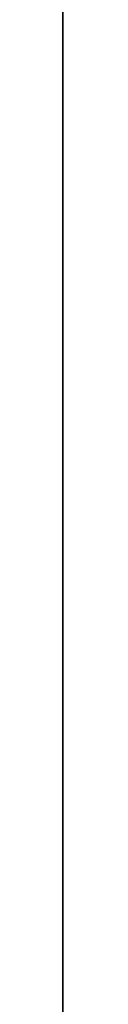
# Model space of a CAD drawing. Units: inches. Extents: x 2083 to 3317, y 1141 to 2115.
# Tile 35 of 256: x 2235.95977 to 2235.95984, y 1477.82142 to 1477.84234. Entities that reach past the tile are written whole.
import ezdxf

# ---------------------------------------------------------------- set-up
doc = ezdxf.new("R2010")
doc.units = ezdxf.units.IN
doc.layers.add('A-ANNO-DIMS', color=2, linetype='Continuous', lineweight=18)
doc.layers.add('A-WALL', color=7, linetype='Continuous', lineweight=35)
doc.layers.add('A-WALL-PATT', color=251, linetype='Continuous', lineweight=13, true_color=0x636466)
doc.styles.get("Standard").update_dxf_attribs({"font": 'arial.ttf'})
doc.dimstyles.new('ISO-25', dxfattribs={"dimtxt": 12, "dimasz": 12, "dimexe": 1.25, "dimexo": 0.625, "dimtad": 1, "dimlunit": 3, "dimtxsty": 'Standard', "dimcen": 2.5, "dimadec": 0, "dimazin": 0, "dimtfac": 1, "dimtmove": 0, "dimatfit": 3, "dimfxl": 1, "dimarcsym": 0})

# ---------------------------------------------------------------- blocks, each defined once
blk = doc.blocks.new('*D30')
at = {"layer": 'A-ANNO-DIMS', "color": 0, "lineweight": -2, "transparency": 16777216}
for p, q in [((2240.017856, 1445.273807), (2240.017856, 1448.045528)), ((2254.329327, 1445.273807), (2254.329327, 1448.045528)), ((2228.017856, 1446.795528), (2216.017856, 1446.795528)), ((2240.017856, 1446.795528), (2254.329327, 1446.795528)), ((2266.329327, 1446.795528), (2413.764866, 1446.795528))]:
    blk.add_line(p, q, dxfattribs=at)
at = {"layer": 'A-ANNO-DIMS', "color": 0, "transparency": 16777216}
for points in [[(2228.017856, 1448.795528), (2228.017856, 1444.795528), (2240.017856, 1446.795528)], [(2266.329327, 1448.795528), (2266.329327, 1444.795528), (2254.329327, 1446.795528)]]:
    blk.add_solid(points, dxfattribs=at)
at = {"layer": 'Defpoints', "color": 0, "transparency": 16777216}
for p in [(2254.329327, 1446.795528), (2240.017856, 1444.648807), (2254.329327, 1444.648807)]:
    blk.add_point(p, dxfattribs=at)
at = {"layer": 'A-ANNO-DIMS', "color": 0, "transparency": 16777216, "insert": (2346.047096, 1453.625167), "char_height": 12, "attachment_point": 5}
blk.add_mtext('WC 1\'-2 1/2" TYP.', dxfattribs=at)
blk = doc.blocks.new('*D31')
at = {"layer": 'A-ANNO-DIMS', "color": 0, "lineweight": -2, "transparency": 16777216}
for p, q in [((2237.871136, 1456.648807), (2237.871136, 1541.915179)), ((2239.392856, 1444.648807), (2236.621136, 1444.648807)), ((2237.871136, 1431.547542), (2237.871136, 1444.648807)), ((2239.392856, 1431.547542), (2236.621136, 1431.547542)), ((2237.871136, 1419.547542), (2237.871136, 1407.547542))]:
    blk.add_line(p, q, dxfattribs=at)
at = {"layer": 'A-ANNO-DIMS', "color": 0, "transparency": 16777216}
for points in [[(2235.871136, 1456.648807), (2239.871136, 1456.648807), (2237.871136, 1444.648807)], [(2235.871136, 1419.547542), (2239.871136, 1419.547542), (2237.871136, 1431.547542)]]:
    blk.add_solid(points, dxfattribs=at)
at = {"layer": 'Defpoints', "color": 0, "transparency": 16777216}
for p in [(2237.871136, 1444.648807), (2240.017856, 1444.648807), (2240.017856, 1431.547542)]:
    blk.add_point(p, dxfattribs=at)
at = {"layer": 'A-ANNO-DIMS', "color": 0, "transparency": 16777216, "insert": (2231.217486, 1505.281993), "char_height": 12, "attachment_point": 5, "rotation": 90}
blk.add_mtext('1\'-1" TYP.', dxfattribs=at)
blk = doc.blocks.new('*D45')
at = {"layer": 'A-ANNO-DIMS', "color": 0, "lineweight": -2, "transparency": 16777216}
for p, q in [((2235.959783, 1478.38636), (2235.959783, 1531.36136)), ((2418.959783, 1478.38636), (2418.959783, 1531.36136)), ((2247.959783, 1530.11136), (2406.959783, 1530.11136))]:
    blk.add_line(p, q, dxfattribs=at)
at = {"layer": 'A-ANNO-DIMS', "color": 0, "transparency": 16777216}
for points in [[(2247.959783, 1532.11136), (2247.959783, 1528.11136), (2235.959783, 1530.11136)], [(2406.959783, 1532.11136), (2406.959783, 1528.11136), (2418.959783, 1530.11136)]]:
    blk.add_solid(points, dxfattribs=at)
at = {"layer": 'Defpoints', "color": 0, "transparency": 16777216}
for p in [(2418.959783, 1530.11136), (2235.959783, 1477.76136), (2418.959783, 1477.76136)]:
    blk.add_point(p, dxfattribs=at)
at = {"layer": 'A-ANNO-DIMS', "color": 0, "transparency": 16777216, "insert": (2327.459783, 1536.867329), "char_height": 12, "attachment_point": 5}
blk.add_mtext('15\'-3"', dxfattribs=at)
blk = doc.blocks.new('*D62')
at = {"layer": 'A-ANNO-DIMS', "color": 0, "lineweight": -2, "transparency": 16777216}
for p, q in [((2235.959783, 1469.38636), (2235.959783, 1522.36136)), ((2379.959783, 1469.38636), (2379.959783, 1522.36136)), ((2247.959783, 1521.11136), (2367.959783, 1521.11136))]:
    blk.add_line(p, q, dxfattribs=at)
at = {"layer": 'A-ANNO-DIMS', "color": 0, "transparency": 16777216}
for points in [[(2247.959783, 1523.11136), (2247.959783, 1519.11136), (2235.959783, 1521.11136)], [(2367.959783, 1523.11136), (2367.959783, 1519.11136), (2379.959783, 1521.11136)]]:
    blk.add_solid(points, dxfattribs=at)
at = {"layer": 'Defpoints', "color": 0, "transparency": 16777216}
for p in [(2379.959783, 1521.11136), (2235.959783, 1468.76136), (2379.959783, 1468.76136)]:
    blk.add_point(p, dxfattribs=at)
at = {"layer": 'A-ANNO-DIMS', "color": 0, "transparency": 16777216, "insert": (2307.959783, 1527.863236), "char_height": 12, "attachment_point": 5}
blk.add_mtext('12\'-0"', dxfattribs=at)

msp = doc.modelspace()

# ---------------------------------------------------------------- hatches: boundary and pattern name
at = {"layer": 'A-WALL-PATT'}
h = msp.add_hatch(color=256, dxfattribs=at)
h.dxf.hatch_style = 1
h.paths.add_polyline_path([(3126.959783, 2020.76136), (2748.959783, 2020.76136), (2604.959783, 2020.76136), (2226.959783, 2020.76136), (2226.959783, 1702.76136), (2466.959783, 1702.76136), (2466.959783, 1582.76136), (2418.959783, 1582.76136), (2418.959783, 1477.76136), (2226.959783, 1477.76136), (2226.959783, 1263.26136), (2544.959783, 1263.26136), (2544.959783, 1411.76136), (2604.959783, 1411.76136), (2685.959783, 1411.76136), (2685.959783, 1420.76136), (2604.959783, 1420.76136), (2604.959783, 1573.76136), (2604.959783, 1702.76136), (2604.959783, 2011.76136), (2748.959783, 2011.76136), (2748.959783, 1702.76136), (2862.959783, 1702.76136), (2862.959783, 1621.76136), (2871.959783, 1621.76136), (2871.959783, 1702.76136), (2883.959783, 1702.76136), (2883.959783, 1706.939459, -0.026459), (2883.959783, 1711.76136), (2757.959783, 1711.76136), (2757.959783, 1807.76136), (2787.959783, 1807.76136), (2787.959783, 1812.26136), (2757.959783, 1812.26136), (2757.959783, 2011.76136), (2877.959783, 2011.76136), (2877.959783, 1812.26136), (2847.959783, 1812.26136), (2847.959783, 1807.76136), (2889.835742, 1807.76136), (2889.835742, 1812.26136), (2882.459783, 1812.26136), (2882.459783, 2011.76136), (3117.959783, 2011.76136), (3117.959783, 1812.26136), (2937.835742, 1812.26136), (2937.835742, 1807.76136), (2995.709783, 1807.76136), (2995.709783, 1796.117666), (3000.209783, 1796.117666), (3000.209783, 1807.76136), (3117.959783, 1807.76136), (3117.959783, 1711.76136), (3000.209783, 1711.76136), (3000.209783, 1760.117666), (2998.572705, 1760.117666, -0.020711), (2995.709783, 1760.117666), (2995.709783, 1711.76136), (2931.959783, 1711.76136), (2931.959783, 1702.76136), (3126.959783, 1702.76136)])
h.paths.add_polyline_path([(2471.459783, 2011.76136), (2471.459783, 1810.01136), (2462.716936, 1810.01136), (2462.716936, 1805.51136), (2505.959783, 1805.51136), (2505.959783, 1810.01136), (2475.959783, 1810.01136), (2475.959783, 2011.76136), (2595.959783, 2011.76136), (2595.959783, 1810.01136), (2565.959783, 1810.01136), (2565.959783, 1805.51136), (2595.959783, 1805.51136), (2595.959783, 1711.76136), (2235.959783, 1711.76136), (2235.959783, 1805.51136), (2353.709783, 1805.51136), (2353.709783, 1796.054162), (2358.209783, 1796.054162), (2358.209783, 1805.51136), (2414.716936, 1805.51136), (2414.716936, 1810.01136), (2235.959783, 1810.01136), (2235.959783, 2011.76136)], flags=16)
h.paths.add_polyline_path([(2270.204734, 1994.610008), (2270.204734, 1970.610008), (2246.204734, 1970.610008), (2246.204734, 1994.610008)], flags=0)
edge = h.paths.add_edge_path(flags=0)
edge.add_ellipse((2332.027391, 1899.798176), major_axis=(-3.042994, 3.042994), ratio=0.16825245, start_angle=-161.332166, end_angle=-156.307114, ccw=False)
edge.add_ellipse((2333.082037, 1898.74353), major_axis=(-1.054646, 1.054646), ratio=0.4535321, start_angle=-123.371019, end_angle=-94.159107)
edge = h.paths.add_edge_path(flags=0)
edge.add_ellipse((2332.027391, 1968.87629), major_axis=(3.042994, 3.042994), ratio=0.16825245, start_angle=18.667834, end_angle=23.692886)
edge.add_spline(control_points=[(2332.925596, 1970.691105), (2332.226768, 1970.3361), (2330.893709, 1969.658905), (2328.41308, 1970.932138), (2327.203934, 1967.748712), (2324.709596, 1969.955589), (2322.532822, 1967.012354), (2320.012846, 1971.295812), (2317.680308, 1968.157845), (2316.040526, 1967.102047), (2315.426904, 1966.809602)], knot_values=[0, 0, 0, 0, 2.267059, 4.324559, 6.685584, 8.878641, 11.121502, 14.300359, 17.755284, 19.732645, 19.732645, 19.732645, 19.732645], degree=3, periodic=0)
edge.add_ellipse((2332.027391, 1968.87629), major_axis=(3.042994, 3.042994), ratio=0.16825245, start_angle=18.667834, end_angle=23.692886, ccw=False)
edge.add_ellipse((2333.082037, 1969.930936), major_axis=(1.054646, 1.054646), ratio=0.4535321, start_angle=56.628981, end_angle=85.840893, ccw=False)
edge = h.paths.add_edge_path(flags=0)
edge.add_spline(control_points=[(2296.428287, 1967.987908), (2293.627804, 1965.336314), (2287.703624, 1959.727094), (2299.74386, 1949.995699), (2294.532591, 1935.668528), (2290.573228, 1920.603512), (2293.394124, 1909.973691), (2296.185407, 1904.966543)], knot_values=[0.099185, 0.099185, 0.099185, 0.099185, 0.345301, 0.619822, 0.982653, 1.386093, 1.810555, 1.810555, 1.810555, 1.810555], degree=3, periodic=0)
edge.add_spline(control_points=[(2296.185407, 1904.966543), (2297.383582, 1902.6193), (2298.000969, 1901.949312), (2298.55297, 1901.468155)], knot_values=[0.006246, 0.006246, 0.006246, 0.006246, 0.055476, 0.055476, 0.055476, 0.055476], degree=3, periodic=0)
edge.add_spline(control_points=[(2298.55297, 1901.468155), (2297.258612, 1900.923224), (2295.225294, 1900.232126), (2293.060229, 1900.614205), (2292.101423, 1900.788415), (2292.089578, 1900.790568)], knot_values=[0.312835, 0.312835, 0.312835, 0.312835, 0.40178, 0.474987, 0.475903, 0.475903, 0.475903, 0.475903], degree=3, periodic=0)
edge.add_arc((2292.793646, 1904.664109), 3.937008, 215.420897, 259.698179, ccw=False)
edge.add_spline(control_points=[(2289.585314, 1902.382304), (2289.476652, 1902.535087), (2289.36848, 1902.688035), (2289.260865, 1902.84117)], knot_values=[0.102872, 0.102872, 0.102872, 0.102872, 0.116896, 0.116896, 0.116896, 0.116896], degree=3, periodic=0)
edge.add_spline(control_points=[(2289.260865, 1902.84117), (2288.686604, 1902.550192), (2287.640048, 1902.019902), (2285.881337, 1901.873954), (2283.852972, 1901.504352), (2281.719987, 1899.710538), (2278.466991, 1899.492942), (2276.157136, 1901.883202), (2272.258953, 1899.804071), (2267.777605, 1901.843183), (2262.243882, 1900.184033), (2257.414927, 1901.782061), (2254.318374, 1900.72612), (2253.178285, 1900.337343)], knot_values=[0, 0, 0, 0, 1.907977, 3.477176, 5.261074, 7.972851, 11.680248, 13.717921, 16.939592, 22.789562, 27.502503, 33.595215, 37.145618, 37.145618, 37.145618, 37.145618], degree=3, periodic=0)
edge.add_line((2253.178285, 1900.337343), (2250.24424, 1902.84117))
edge.add_line((2250.24424, 1902.84117), (2250.24424, 1965.833296))
edge.add_line((2250.24424, 1965.833296), (2253.178285, 1968.337123))
edge.add_spline(control_points=[(2253.178285, 1968.337123), (2254.318374, 1967.948346), (2257.414927, 1966.892405), (2262.243882, 1968.490433), (2267.777605, 1966.831283), (2271.52673, 1968.537217), (2273.875914, 1967.828289), (2274.206701, 1967.727642)], knot_values=[0, 0, 0, 0, 0.09018, 0.244935, 0.364644, 0.513233, 0.537855, 0.537855, 0.537855, 0.537855], degree=3, periodic=0)
edge.add_arc((2274.352887, 1963.793349), 3.937008, 72.051134, 92.127949, ccw=False)
edge.add_arc((2281.296933, 1985.230003), 18.596298, 252.0511336, 288.5657217)
edge.add_arc((2292.316717, 1956.02888), 12.646081, 71.0267879, 113.7782184, ccw=False)
edge = h.paths.add_edge_path(flags=0)
edge.add_spline(control_points=[(2274.899415, 1951.856195), (2275.066156, 1951.616592), (2275.232687, 1951.376588), (2275.397987, 1951.135855)], knot_values=[1.409916, 1.409916, 1.409916, 1.409916, 1.43159, 1.43159, 1.43159, 1.43159], degree=3, periodic=0)
edge.add_spline(control_points=[(2275.397987, 1951.135855), (2275.792106, 1950.561885), (2276.179231, 1949.983774), (2276.545546, 1949.397103)], knot_values=[1.358238, 1.358238, 1.358238, 1.358238, 1.409916, 1.409916, 1.409916, 1.409916], degree=3, periodic=0)
edge.add_line((2276.545546, 1949.397103), (2277.437289, 1947.862185))
edge.add_spline(control_points=[(2277.437289, 1947.862185), (2276.303834, 1945.673115), (2274.639698, 1942.426882), (2274.631615, 1938.0939), (2272.799124, 1930.85155), (2274.356426, 1943.897046), (2275.947681, 1947.923356), (2276.545546, 1949.397103)], knot_values=[0.005632, 0.005632, 0.005632, 0.005632, 0.186014, 0.266002, 0.357087, 0.59639, 0.739732, 0.739732, 0.739732, 0.739732], degree=3, periodic=0)
edge.add_spline(control_points=[(2276.545546, 1949.397103), (2276.179231, 1949.983774), (2275.792106, 1950.561885), (2275.397987, 1951.135855)], knot_values=[1.358238, 1.358238, 1.358238, 1.358238, 1.409916, 1.409916, 1.409916, 1.409916], degree=3, periodic=0)
edge.add_spline(control_points=[(2275.397987, 1951.135855), (2274.9425, 1950.080452), (2274.20776, 1948.025272), (2273.934602, 1944.851477), (2272.468534, 1937.627489), (2273.466216, 1945.696466), (2274.700615, 1951.059472), (2274.899415, 1951.856195)], knot_values=[0.104364, 0.104364, 0.104364, 0.104364, 0.189636, 0.269624, 0.36071, 0.600013, 0.644622, 0.644622, 0.644622, 0.644622], degree=3, periodic=0)
h.paths.add_polyline_path([(2269.167514, 1963.127573, -0.357527), (2268.170633, 1960.97637, -0.092561), (2268.170633, 1939.436325, -0.357527), (2269.167514, 1937.285122, -0.357527), (2267.01631, 1938.282002, -0.164785), (2254.685581, 1938.282002, -0.357527), (2252.534378, 1937.285122, -0.357527), (2253.531259, 1939.436325, -0.092561), (2253.531259, 1960.97637, -0.357527), (2252.534378, 1963.127573, -0.357527), (2254.685581, 1962.130692, -0.164785), (2267.01631, 1962.130692, -0.357527)], flags=0)
h.paths.add_polyline_path([(2248.874068, 1967.8018), (2248.874068, 1957.02771), (2249.457783, 1957.02771), (2249.457783, 1911.646756), (2248.874068, 1911.646756), (2248.874068, 1900.872666), (2246.511863, 1900.872666, 0.197327), (2244.149658, 1902.456873), (2244.149658, 1966.217592, 0.197327), (2246.511863, 1967.8018)], flags=0)
h.paths.add_polyline_path([(2269.167514, 1931.389344, -0.357527), (2268.170633, 1929.238141, -0.092561), (2268.170633, 1907.698096, -0.357527), (2269.167514, 1905.546893, -0.357527), (2267.01631, 1906.543774, -0.164785), (2254.685581, 1906.543774, -0.357527), (2252.534378, 1905.546893, -0.357527), (2253.531259, 1907.698096, -0.092561), (2253.531259, 1929.238141, -0.357527), (2252.534378, 1931.389344, -0.357527), (2254.685581, 1930.392463, -0.164785), (2267.01631, 1930.392463, -0.357527)], flags=0)
edge = h.paths.add_edge_path(flags=0)
edge.add_spline(control_points=[(2276.196858, 1906.723702), (2276.168144, 1909.028928), (2276.114049, 1913.371852), (2270.598417, 1924.924978), (2273.905175, 1919.012779), (2275.921711, 1916.262063), (2275.47457, 1912.402149), (2277.257874, 1910.380621), (2276.696044, 1908.225036), (2276.646218, 1906.813023), (2276.617825, 1906.008407)], knot_values=[0, 0, 0, 0, 8.61026, 16.221274, 18.843057, 23.804898, 27.440828, 29.356102, 31.203478, 33.650687, 33.650687, 33.650687, 33.650687], degree=3, periodic=0)
edge.add_spline(control_points=[(2276.617825, 1906.008407), (2276.623313, 1905.624144), (2276.497738, 1904.628661), (2275.441779, 1903.854725), (2274.937314, 1903.08045), (2274.85908, 1902.84117)], knot_values=[0.156488, 0.156488, 0.156488, 0.156488, 0.184398, 0.231376, 0.250598, 0.250598, 0.250598, 0.250598], degree=3, periodic=0)
edge.add_line((2274.85908, 1902.84117), (2276.50598, 1902.84117))
edge.add_spline(control_points=[(2276.50598, 1902.84117), (2276.788308, 1903.08494), (2277.665071, 1904.125196), (2278.249538, 1904.340738), (2277.653872, 1908.527387), (2278.15567, 1906.227808), (2278.100464, 1905.285948), (2278.846675, 1904.069005), (2277.856785, 1903.414948), (2277.874191, 1902.99105), (2277.903562, 1902.84117)], knot_values=[0.059574, 0.059574, 0.059574, 0.059574, 0.080753, 0.103741, 0.16972, 0.176036, 0.207137, 0.240474, 0.262341, 0.27366, 0.27366, 0.27366, 0.27366], degree=3, periodic=0)
edge.add_line((2277.903562, 1902.84117), (2280.029825, 1902.84117))
edge.add_spline(control_points=[(2280.029825, 1902.84117), (2279.888221, 1903.088398), (2279.499257, 1903.981551), (2280.152284, 1905.939349), (2278.103615, 1909.657757), (2279.762395, 1907.185285), (2280.3279, 1904.874861), (2280.485109, 1903.48959), (2281.463269, 1903.249432), (2281.758343, 1902.936497), (2281.834036, 1902.84117)], knot_values=[0.013856, 0.013856, 0.013856, 0.013856, 0.034874, 0.088867, 0.107879, 0.126738, 0.158714, 0.193757, 0.217487, 0.226722, 0.226722, 0.226722, 0.226722], degree=3, periodic=0)
edge.add_spline(control_points=[(2281.834036, 1902.84117), (2281.787535, 1902.826703), (2281.647022, 1902.782988), (2281.395527, 1902.85949), (2281.088077, 1902.985242), (2280.720683, 1903.060902), (2280.333451, 1903.025726), (2280.124767, 1902.898879), (2280.029825, 1902.84117)], knot_values=[0, 0, 0, 0, 0.14413, 0.435517, 0.749276, 1.153046, 1.548371, 1.878348, 1.878348, 1.878348, 1.878348], degree=3, periodic=0)
edge.add_line((2280.029825, 1902.84117), (2277.903562, 1902.84117))
edge.add_spline(control_points=[(2277.903562, 1902.84117), (2277.892855, 1902.795855), (2277.865396, 1902.679637), (2277.607479, 1902.687483), (2277.27405, 1902.8007), (2276.837921, 1902.619775), (2276.583807, 1902.789261), (2276.50598, 1902.84117)], knot_values=[0, 0, 0, 0, 0.127189, 0.326199, 0.628009, 1.24357, 1.515331, 1.515331, 1.515331, 1.515331], degree=3, periodic=0)
edge.add_line((2276.50598, 1902.84117), (2274.85908, 1902.84117))
edge.add_spline(control_points=[(2274.85908, 1902.84117), (2274.814437, 1902.898587), (2274.72513, 1903.013446), (2274.493477, 1903.118968), (2274.244285, 1902.960539), (2273.937121, 1903.184942), (2273.614039, 1902.983143), (2273.408316, 1902.883045), (2273.322254, 1902.84117)], knot_values=[0, 0, 0, 0, 0.21843, 0.436957, 0.687977, 0.990379, 1.398396, 1.69185, 1.69185, 1.69185, 1.69185], degree=3, periodic=0)
edge.add_spline(control_points=[(2273.322254, 1902.84117), (2273.61674, 1903.445692), (2274.273998, 1904.538253), (2276.027239, 1904.573702), (2276.206963, 1906.583637), (2276.196858, 1906.723702)], knot_values=[0.012227, 0.012227, 0.012227, 0.012227, 0.059472, 0.106218, 0.134458, 0.134458, 0.134458, 0.134458], degree=3, periodic=0)
h.paths.add_polyline_path([(2270.776054, 1897.789828), (2270.776054, 1873.789828), (2246.776054, 1873.789828), (2246.776054, 1897.789828)], flags=0)
h.paths.add_polyline_path([(2353.709783, 1760.005059), (2353.709783, 1760.054162), (2358.209783, 1760.054162, -0.033729)], flags=0)
h.paths.add_polyline_path([(2321.819119, 1737.529186), (2341.995327, 1737.529186, -0.414214), (2343.203273, 1736.321241), (2343.203273, 1721.020596, -0.414214), (2341.995327, 1719.812651), (2321.819119, 1719.812651, -0.414214), (2320.611173, 1721.020596), (2320.611173, 1736.321241, -0.414214)], flags=0)
h.paths.add_polyline_path([(2324.23501, 1736.321241), (2339.579436, 1736.321241, -0.414214), (2341.995327, 1733.905349), (2341.995327, 1725.44973, -0.414214), (2339.579436, 1723.033839), (2333.680588, 1723.033839), (2333.845317, 1722.045467, -0.870646), (2335.425399, 1721.825893, -0.767327), (2333.922694, 1721.423245), (2331.291024, 1721.423245, -0.767327), (2329.788319, 1721.825893, -0.870646), (2331.368401, 1722.045467), (2331.53313, 1723.033839), (2324.23501, 1723.033839, -0.414214), (2321.819119, 1725.44973), (2321.819119, 1733.905349, -0.414214)], flags=0)
h.paths.add_polyline_path([(2570.483789, 1928.615444), (2589.683789, 1928.615444), (2590.168829, 1928.615444), (2590.168829, 1904.993397), (2570.483789, 1904.993397)], flags=0)
h.paths.add_polyline_path([(2574.447324, 1927.263822, -1), (2572.828836, 1927.263822, -1)], flags=0)
h.paths.add_polyline_path([(2573.089867, 1926.940877), (2573.925032, 1927.776042), (2574.147743, 1927.553332), (2573.312577, 1926.718166)], flags=0)
h.paths.add_polyline_path([(2578.779065, 1919.729618, -1), (2571.591663, 1919.729618, -1)], flags=0)
h.paths.add_polyline_path([(2578.385364, 1919.729618, -1), (2571.985364, 1919.729618, -1)], flags=0)
h.paths.add_polyline_path([(2331.595764, 1729.476216, -1), (2333.617954, 1729.476216, -1)], flags=0)
h.paths.add_polyline_path([(2578.034228, 1927.263822, -1), (2576.41574, 1927.263822, -1)], flags=0)
h.paths.add_polyline_path([(2576.688851, 1927.531089), (2576.911562, 1927.753799), (2577.746728, 1926.918634), (2577.524017, 1926.695923)], flags=0)
h.paths.add_polyline_path([(2578.139065, 1909.859539, -1), (2572.231663, 1909.859539, -1)], flags=0)
h.paths.add_polyline_path([(2577.745364, 1909.859539, -1), (2572.625364, 1909.859539, -1)], flags=0)
h.paths.add_polyline_path([(2583.797718, 1927.263822, -1), (2582.179229, 1927.263822, -1)], flags=0)
h.paths.add_polyline_path([(2582.718649, 1927.753799), (2583.553814, 1926.918634), (2583.331103, 1926.695923), (2582.495938, 1927.531089)], flags=0)
h.paths.add_polyline_path([(2582.495938, 1927.531089), (2582.718649, 1927.753799), (2583.553814, 1926.918634), (2583.331103, 1926.695923)], flags=0)
h.paths.add_polyline_path([(2587.739065, 1920.529618, -1), (2581.831663, 1920.529618, -1)], flags=0)
h.paths.add_polyline_path([(2587.345364, 1920.529618, -1), (2582.225364, 1920.529618, -1)], flags=0)
h.paths.add_polyline_path([(2587.384622, 1927.263822, -1), (2585.766133, 1927.263822, -1)], flags=0)
h.paths.add_polyline_path([(2586.081993, 1926.980247), (2586.917158, 1927.815412), (2587.139869, 1927.592702), (2586.304703, 1926.757536)], flags=0)
h.paths.add_polyline_path([(2588.379065, 1910.659539, -1), (2581.191663, 1910.659539, -1)], flags=0)
h.paths.add_polyline_path([(2587.985364, 1910.659539, -1), (2581.585364, 1910.659539, -1)], flags=0)
h.paths.add_polyline_path([(2417.167729, 1729.477895), (2437.343937, 1729.477895, -0.414214), (2438.551883, 1728.26995), (2438.551883, 1712.969306, -0.414214), (2437.343937, 1711.76136), (2417.167729, 1711.76136, -0.414214), (2415.959783, 1712.969306), (2415.959783, 1728.26995, -0.414214)], flags=0)
h.paths.add_polyline_path([(2419.58362, 1728.26995), (2434.928046, 1728.26995, -0.414214), (2437.343937, 1725.854059), (2437.343937, 1717.39844, -0.414214), (2434.928046, 1714.982548), (2429.029199, 1714.982548), (2429.193927, 1713.994176, -0.870646), (2430.774009, 1713.774603, -0.767327), (2429.271304, 1713.371954), (2426.639634, 1713.371954, -0.767327), (2425.136929, 1713.774603, -0.870646), (2426.717011, 1713.994176), (2426.88174, 1714.982548), (2419.58362, 1714.982548, -0.414214), (2417.167729, 1717.39844), (2417.167729, 1725.854059, -0.414214)], flags=0)
h.paths.add_polyline_path([(2419.58362, 1728.26995), (2434.928046, 1728.26995, -0.414214), (2437.343937, 1725.854059), (2437.343937, 1717.39844, -0.414214), (2434.928046, 1714.982548), (2429.029199, 1714.982548), (2428.358118, 1719.009034), (2427.552821, 1719.009034), (2426.88174, 1714.982548), (2419.58362, 1714.982548, -0.414214), (2417.167729, 1717.39844), (2417.167729, 1725.854059, -0.414214)], flags=0)
h.paths.add_polyline_path([(2426.944374, 1721.424925, -1), (2428.966564, 1721.424925, -1)], flags=0)
h.paths.add_polyline_path([(2475.959783, 1702.76136), (2595.959783, 1702.76136), (2595.959783, 1582.76136), (2475.959783, 1582.76136)], flags=16)
h.paths.add_polyline_path([(2427.959783, 1573.76136), (2595.959783, 1573.76136), (2595.959783, 1468.76136), (2595.959783, 1420.76136), (2384.459783, 1420.76136), (2384.459783, 1468.76136), (2427.959783, 1468.76136)], flags=16)
h.paths.add_polyline_path([(2379.959783, 1468.76136), (2379.959783, 1420.76136), (2235.959783, 1420.76136), (2235.959783, 1468.76136)], flags=16)
h.paths.add_polyline_path([(2317.815996, 1466.695767), (2337.992205, 1466.695767, -0.414214), (2339.20015, 1465.487821), (2339.20015, 1450.187177, -0.414214), (2337.992205, 1448.979232), (2317.815996, 1448.979232, -0.414214), (2316.608051, 1450.187177), (2316.608051, 1465.487821, -0.414214)], flags=0)
h.paths.add_polyline_path([(2320.231887, 1465.487821), (2335.576313, 1465.487821, -0.414214), (2337.992205, 1463.07193), (2337.992205, 1454.616311, -0.414214), (2335.576313, 1452.20042), (2329.677466, 1452.20042), (2329.842195, 1451.212047, -0.870646), (2331.422276, 1450.992474, -0.767327), (2329.919571, 1450.589826), (2327.287902, 1450.589826, -0.767327), (2325.785197, 1450.992474, -0.870646), (2327.365278, 1451.212047), (2327.530007, 1452.20042), (2320.231887, 1452.20042, -0.414214), (2317.815996, 1454.616311), (2317.815996, 1463.07193, -0.414214)], flags=0)
h.paths.add_polyline_path([(2320.231887, 1465.487821), (2335.576313, 1465.487821, -0.414214), (2337.992205, 1463.07193), (2337.992205, 1454.616311, -0.414214), (2335.576313, 1452.20042), (2329.677466, 1452.20042), (2329.006385, 1456.226905), (2328.201088, 1456.226905), (2327.530007, 1452.20042), (2320.231887, 1452.20042, -0.414214), (2317.815996, 1454.616311), (2317.815996, 1463.07193, -0.414214)], flags=0)
h.paths.add_polyline_path([(2327.592641, 1458.642796, -1), (2329.614832, 1458.642796, -1)], flags=0)
h.paths.add_polyline_path([(2244.411744, 1433.340453), (2241.920945, 1433.340453, -0.414214), (2240.017856, 1435.243542), (2240.017856, 1440.952808, -0.414211), (2241.920925, 1442.855897), (2244.411744, 1442.855897, -1.976472)], flags=0)
h.paths.add_polyline_path([(2245.356888, 1434.397536, -0.414214), (2245.356888, 1441.798814, -2.144098)], flags=0)
h.paths.add_polyline_path([(2535.959783, 1416.26136), (2535.959783, 1272.26136), (2235.959783, 1272.26136), (2235.959783, 1416.26136)], flags=16)
h.paths.add_polyline_path([(2260.119561, 1384.292841), (2260.119561, 1362.038649), (2237.865369, 1362.038649), (2237.865369, 1384.292841)], flags=0)
edge = h.paths.add_edge_path(flags=0)
edge.add_line((2318.251847, 1362.093298), (2318.145797, 1362.000973))
edge.add_ellipse((2317.445116, 1360.431044), major_axis=(2.82164, 2.82164), ratio=0.16825245, start_angle=18.667834, end_angle=20.948127, ccw=False)
edge.add_ellipse((2318.423045, 1361.408974), major_axis=(0.977929, 0.977929), ratio=0.4535321, start_angle=56.628981, end_angle=70.226201, ccw=False)
edge = h.paths.add_edge_path(flags=0)
edge.add_line((2319.10737, 1295.571078), (2319.015044, 1295.677128))
edge.add_ellipse((2317.445116, 1296.377809), major_axis=(-2.82164, 2.82164), ratio=0.16825245, start_angle=-161.332166, end_angle=-159.051873, ccw=False)
edge.add_ellipse((2318.423045, 1295.39988), major_axis=(-0.977929, 0.977929), ratio=0.4535321, start_angle=-123.371019, end_angle=-109.773799)
edge = h.paths.add_edge_path(flags=0)
edge.add_spline(control_points=[(2284.210349, 1301.170219), (2284.580688, 1300.444719), (2284.891189, 1299.892024), (2285.159553, 1299.461018)], knot_values=[0.039066, 0.039066, 0.039066, 0.039066, 0.055476, 0.055476, 0.055476, 0.055476], degree=3, periodic=0)
edge.add_line((2285.159553, 1299.461018), (2284.210349, 1301.170219))
edge = h.paths.add_edge_path(flags=0)
edge.add_line((2280.412458, 1297.298013), (2283.369991, 1297.036122))
edge.add_line((2283.369991, 1297.036122), (2286.40569, 1297.92631))
edge.add_spline(control_points=[(2286.40569, 1297.92631), (2285.305487, 1297.463119), (2284.344777, 1297.129151), (2283.369991, 1297.036122)], knot_values=[0.394369, 0.394369, 0.394369, 0.394369, 0.475903, 0.475903, 0.475903, 0.475903], degree=3, periodic=0)
edge.add_spline(control_points=[(2283.369991, 1297.036122), (2283.28139, 1297.027666), (2282.316289, 1296.957336), (2281.312502, 1297.134479), (2280.423441, 1297.296016), (2280.412458, 1297.298013)], knot_values=[0.312835, 0.312835, 0.312835, 0.312835, 0.320246, 0.393453, 0.394369, 0.394369, 0.394369, 0.394369], degree=3, periodic=0)
edge = h.paths.add_edge_path(flags=0)
edge.add_line((2284.435561, 1359.607285), (2280.446291, 1355.328047))
edge.add_line((2280.446291, 1355.328047), (2279.579987, 1351.017754))
edge.add_line((2279.579987, 1351.017754), (2282.412974, 1346.580433))
edge.add_spline(control_points=[(2282.412974, 1346.580433), (2283.153331, 1345.589236), (2284.252896, 1344.028897), (2284.801037, 1342.387167), (2284.935162, 1341.805544)], knot_values=[1.240098, 1.240098, 1.240098, 1.240098, 1.332892, 1.382712, 1.382712, 1.382712, 1.382712], degree=3, periodic=0)
edge.add_spline(control_points=[(2284.935162, 1341.805544), (2285.319108, 1340.1406), (2285.233029, 1338.409204), (2284.909938, 1336.654122)], knot_values=[1.097484, 1.097484, 1.097484, 1.097484, 1.240098, 1.240098, 1.240098, 1.240098], degree=3, periodic=0)
edge.add_spline(control_points=[(2284.909938, 1336.654122), (2284.586848, 1334.89904), (2284.026745, 1333.120272), (2283.462644, 1331.360585)], knot_values=[0.95487, 0.95487, 0.95487, 0.95487, 1.097484, 1.097484, 1.097484, 1.097484], degree=3, periodic=0)
edge.add_line((2283.462644, 1331.360585), (2281.890376, 1326.153357))
edge.add_line((2281.890376, 1326.153357), (2280.756259, 1321.056089))
edge.add_line((2280.756259, 1321.056089), (2280.299205, 1316.001977))
edge.add_line((2280.299205, 1316.001977), (2280.715933, 1310.950068))
edge.add_line((2280.715933, 1310.950068), (2282.028094, 1305.972137))
edge.add_line((2282.028094, 1305.972137), (2284.210349, 1301.170219))
edge.add_spline(control_points=[(2284.210349, 1301.170219), (2283.340731, 1302.730185), (2282.611904, 1304.336493), (2282.028094, 1305.972137)], knot_values=[0.099185, 0.099185, 0.099185, 0.099185, 0.241799, 0.241799, 0.241799, 0.241799], degree=3, periodic=0)
edge.add_spline(control_points=[(2282.028094, 1305.972137), (2281.444283, 1307.60778), (2281.005489, 1309.272759), (2280.715933, 1310.950068)], knot_values=[0.241799, 0.241799, 0.241799, 0.241799, 0.384413, 0.384413, 0.384413, 0.384413], degree=3, periodic=0)
edge.add_spline(control_points=[(2280.715933, 1310.950068), (2280.433241, 1312.587613), (2280.289386, 1314.276959), (2280.298894, 1315.962032), (2280.299205, 1316.001977)], knot_values=[0.384413, 0.384413, 0.384413, 0.384413, 0.523647, 0.527028, 0.527028, 0.527028, 0.527028], degree=3, periodic=0)
edge.add_spline(control_points=[(2280.299205, 1316.001977), (2280.312326, 1317.686955), (2280.477871, 1319.367926), (2280.756259, 1321.056089)], knot_values=[0.527028, 0.527028, 0.527028, 0.527028, 0.669642, 0.669642, 0.669642, 0.669642], degree=3, periodic=0)
edge.add_spline(control_points=[(2280.756259, 1321.056089), (2281.034648, 1322.744252), (2281.42588, 1324.439608), (2281.890376, 1326.153357)], knot_values=[0.669642, 0.669642, 0.669642, 0.669642, 0.812256, 0.812256, 0.812256, 0.812256], degree=3, periodic=0)
edge.add_spline(control_points=[(2281.890376, 1326.153357), (2282.264383, 1327.533251), (2282.78787, 1329.26181), (2283.352751, 1331.01778), (2283.462644, 1331.360585)], knot_values=[0.812256, 0.812256, 0.812256, 0.812256, 0.927087, 0.95487, 0.95487, 0.95487, 0.95487], degree=3, periodic=0)
edge.add_line((2283.462644, 1331.360585), (2284.909938, 1336.654122))
edge.add_line((2284.909938, 1336.654122), (2284.935162, 1341.805544))
edge.add_line((2284.935162, 1341.805544), (2282.412974, 1346.580433))
edge.add_spline(control_points=[(2282.412974, 1346.580433), (2281.275127, 1348.103792), (2280.078447, 1349.570318), (2279.579987, 1351.017754)], knot_values=[1.382712, 1.382712, 1.382712, 1.382712, 1.525326, 1.525326, 1.525326, 1.525326], degree=3, periodic=0)
edge.add_spline(control_points=[(2279.579987, 1351.017754), (2279.443282, 1351.414721), (2279.136312, 1352.856922), (2279.73519, 1354.290385), (2280.446291, 1355.328047)], knot_values=[1.525326, 1.525326, 1.525326, 1.525326, 1.564439, 1.667941, 1.667941, 1.667941, 1.667941], degree=3, periodic=0)
edge.add_spline(control_points=[(2280.446291, 1355.328047), (2281.426113, 1356.757835), (2282.930837, 1358.18256), (2284.435561, 1359.607285)], knot_values=[1.667941, 1.667941, 1.667941, 1.667941, 1.810555, 1.810555, 1.810555, 1.810555], degree=3, periodic=0)
edge.add_arc((2280.623075, 1348.518181), 11.72618, 71.0267879, 113.7782184)
edge.add_arc((2270.404892, 1375.595156), 17.243567, 252.0511336, 288.5657217, ccw=False)
edge.add_arc((2263.965969, 1355.717847), 3.650622, 72.051134, 92.127949)
edge.add_arc((2263.965969, 1355.717847), 3.650622, 92.127949, 177.98513)
edge.add_spline(control_points=[(2260.317604, 1355.846199), (2260.260417, 1354.220668), (2260.551278, 1350.186547), (2262.999344, 1346.766251), (2264.472741, 1344.649024)], knot_values=[1.43159, 1.43159, 1.43159, 1.43159, 1.564144, 1.770695, 1.770695, 1.770695, 1.770695], degree=3, periodic=0)
edge.add_line((2264.472741, 1344.649024), (2264.93559, 1343.98253))
edge.add_spline(control_points=[(2263.801044, 1340.248105), (2263.843238, 1340.514088), (2264.067244, 1341.756465), (2264.512693, 1343.002453), (2264.935047, 1343.981083)], knot_values=[0.53657, 0.53657, 0.53657, 0.53657, 0.559349, 0.644622, 0.644622, 0.644622, 0.644622], degree=3, periodic=0)
edge.add_spline(control_points=[(2264.935047, 1343.981083), (2265.117771, 1343.714975), (2265.298875, 1343.447906), (2265.476756, 1343.179365)], knot_values=[1.384077, 1.384077, 1.384077, 1.384077, 1.409916, 1.409916, 1.409916, 1.409916], degree=3, periodic=0)
edge.add_spline(control_points=[(2265.476756, 1343.179365), (2265.654637, 1342.910823), (2265.829296, 1342.64081), (2265.99913, 1342.368812)], knot_values=[1.358238, 1.358238, 1.358238, 1.358238, 1.384077, 1.384077, 1.384077, 1.384077], degree=3, periodic=0)
edge.add_line((2265.99913, 1342.368812), (2266.826006, 1340.945547))
edge.add_spline(control_points=[(2266.826006, 1340.945547), (2268.894401, 1337.089691), (2271.398173, 1325.843001), (2270.516164, 1310.568557), (2275.919376, 1301.860609), (2277.789511, 1299.19945)], knot_values=[0.116896, 0.116896, 0.116896, 0.116896, 0.472987, 1.050969, 1.313793, 1.313793, 1.313793, 1.313793], degree=3, periodic=0)
edge.add_spline(control_points=[(2277.789511, 1299.19945), (2277.839405, 1299.128452), (2277.889428, 1299.057498), (2277.939572, 1298.986584)], knot_values=[0.109884, 0.109884, 0.109884, 0.109884, 0.116896, 0.116896, 0.116896, 0.116896], degree=3, periodic=0)
edge.add_line((2277.939572, 1298.986584), (2277.788849, 1299.199114))
edge.add_spline(control_points=[(2277.788849, 1299.199114), (2277.256582, 1298.929414), (2276.28635, 1298.437902), (2275.039352, 1298.334419), (2274.38333, 1298.238895), (2274.215254, 1298.209338)], knot_values=[33.12187, 33.12187, 33.12187, 33.12187, 35.029056, 36.598255, 37.144827, 37.144827, 37.144827, 37.144827], degree=3, periodic=0)
edge.add_line((2274.215254, 1298.209338), (2273.073147, 1297.892961))
edge.add_spline(control_points=[(2273.073147, 1297.892961), (2272.322936, 1297.579784), (2271.039151, 1296.510508), (2269.248395, 1296.226062), (2268.4231, 1296.374654)], knot_values=[26.532584, 26.532584, 26.532584, 26.532584, 29.198919, 31.839101, 31.839101, 31.839101, 31.839101], degree=3, periodic=0)
edge.add_line((2268.4231, 1296.374654), (2263.878501, 1297.457534))
edge.add_spline(control_points=[(2263.878501, 1297.457534), (2263.556077, 1297.359435), (2261.860306, 1296.838694), (2260.23878, 1297.282407), (2258.933454, 1297.516461)], knot_values=[15.919551, 15.919551, 15.919551, 15.919551, 16.939592, 21.226067, 21.226067, 21.226067, 21.226067], degree=3, periodic=0)
edge.add_line((2258.933454, 1297.516461), (2254.055233, 1297.32901))
edge.add_spline(control_points=[(2254.055233, 1297.32901), (2253.755525, 1297.295815), (2252.113683, 1297.165174), (2250.461869, 1297.544221), (2249.129686, 1297.667882)], knot_values=[5.306517, 5.306517, 5.306517, 5.306517, 6.276435, 10.613034, 10.613034, 10.613034, 10.613034], degree=3, periodic=0)
edge.add_line((2249.129686, 1297.667882), (2244.33165, 1296.877756))
edge.add_line((2244.33165, 1296.877756), (2241.611033, 1299.19945))
edge.add_line((2241.611033, 1299.19945), (2241.611033, 1357.609404))
edge.add_line((2241.611033, 1357.609404), (2244.33165, 1359.931097))
edge.add_line((2244.33165, 1359.931097), (2252.728823, 1359.542692))
edge.add_spline(control_points=[(2252.728823, 1359.542692), (2252.870939, 1359.54644), (2253.30574, 1359.548172), (2253.739845, 1359.514274), (2254.031742, 1359.482426)], knot_values=[0.233291, 0.233291, 0.233291, 0.233291, 0.244935, 0.268927, 0.268927, 0.268927, 0.268927], degree=3, periodic=0)
edge.add_line((2254.031742, 1359.482426), (2259.58719, 1359.41639))
edge.add_spline(control_points=[(2259.58719, 1359.41639), (2260.677068, 1359.628503), (2262.073197, 1359.897003), (2263.523692, 1359.459278), (2263.830417, 1359.365952)], knot_values=[0.422516, 0.422516, 0.422516, 0.422516, 0.513233, 0.537855, 0.537855, 0.537855, 0.537855], degree=3, periodic=0)
edge.add_arc((2263.965969, 1355.717847), 3.650622, 72.051134, 92.127949, ccw=False)
edge.add_arc((2270.404892, 1375.595156), 17.243567, 252.0511336, 288.5657217)
edge.add_arc((2280.623075, 1348.518181), 11.72618, 71.0267879, 113.7782184, ccw=False)
h.paths.add_polyline_path([(2240.34053, 1359.434715), (2240.34053, 1349.444353), (2240.881785, 1349.444353), (2240.881785, 1307.3645), (2240.34053, 1307.3645), (2240.34053, 1297.374138), (2238.150157, 1297.374138, 0.197327), (2235.959783, 1298.843108), (2235.959783, 1357.965746, 0.197327), (2238.150157, 1359.434715)], flags=0)
h.paths.add_polyline_path([(2259.15779, 1355.1005, -0.357527), (2258.233425, 1353.10578, -0.092561), (2258.233425, 1333.132601, -0.357527), (2259.15779, 1331.13788, -0.357527), (2257.16307, 1332.062246, -0.164785), (2245.729302, 1332.062246, -0.357527), (2243.734582, 1331.13788, -0.357527), (2244.658947, 1333.132601, -0.092561), (2244.658947, 1353.10578, -0.357527), (2243.734582, 1355.1005, -0.357527), (2245.729302, 1354.176135, -0.164785), (2257.16307, 1354.176135, -0.357527)], flags=0)
edge = h.paths.add_edge_path(flags=0)
edge.add_line((2265.99913, 1342.368812), (2266.826006, 1340.945547))
edge.add_line((2266.826006, 1340.945547), (2265.307557, 1337.814066))
edge.add_line((2265.307557, 1337.814066), (2264.358232, 1334.652939))
edge.add_line((2264.358232, 1334.652939), (2264.262012, 1333.799705))
edge.add_spline(control_points=[(2264.262012, 1333.799705), (2264.208357, 1333.187055), (2264.16206, 1332.365525), (2264.007144, 1331.413933), (2263.969049, 1331.201834)], knot_values=[0.464444, 0.464444, 0.464444, 0.464444, 0.516691, 0.531608, 0.531608, 0.531608, 0.531608], degree=3, periodic=0)
edge.add_spline(control_points=[(2263.969049, 1331.201834), (2263.774535, 1330.118873), (2263.42437, 1328.790839), (2263.25742, 1328.530652), (2263.234028, 1328.514612)], knot_values=[0.372682, 0.372682, 0.372682, 0.372682, 0.44885, 0.464444, 0.464444, 0.464444, 0.464444], degree=3, periodic=0)
edge.add_spline(control_points=[(2263.234028, 1328.514612), (2263.096382, 1328.420227), (2263.13117, 1329.301477), (2263.274953, 1330.615749)], knot_values=[0.280919, 0.280919, 0.280919, 0.280919, 0.372682, 0.372682, 0.372682, 0.372682], degree=3, periodic=0)
edge.add_spline(control_points=[(2263.274953, 1330.615749), (2263.418736, 1331.930022), (2263.671515, 1333.677318), (2263.969852, 1335.315027)], knot_values=[0.189157, 0.189157, 0.189157, 0.189157, 0.280919, 0.280919, 0.280919, 0.280919], degree=3, periodic=0)
edge.add_spline(control_points=[(2263.969852, 1335.315027), (2264.100496, 1336.032192), (2264.418783, 1337.621911), (2264.754848, 1338.86443), (2264.947419, 1339.491124)], knot_values=[0.097394, 0.097394, 0.097394, 0.097394, 0.137578, 0.189157, 0.189157, 0.189157, 0.189157], degree=3, periodic=0)
edge.add_spline(control_points=[(2264.947419, 1339.491124), (2265.290017, 1340.606055), (2265.644238, 1341.493996), (2265.99913, 1342.368812)], knot_values=[0.005632, 0.005632, 0.005632, 0.005632, 0.097394, 0.097394, 0.097394, 0.097394], degree=3, periodic=0)
h.paths.add_polyline_path([(2259.15779, 1325.670973, -0.357527), (2258.233425, 1323.676253, -0.092561), (2258.233425, 1303.703073, -0.357527), (2259.15779, 1301.708353, -0.357527), (2257.16307, 1302.632719, -0.164785), (2245.729302, 1302.632719, -0.357527), (2243.734582, 1301.708353, -0.357527), (2244.658947, 1303.703073, -0.092561), (2244.658947, 1323.676253, -0.357527), (2243.734582, 1325.670973, -0.357527), (2245.729302, 1324.746608, -0.164785), (2257.16307, 1324.746608, -0.357527)], flags=0)
edge = h.paths.add_edge_path(flags=0)
edge.add_spline(control_points=[(2261.708938, 1317.311421), (2261.679482, 1317.41758), (2261.761858, 1317.388535), (2262.490736, 1316.089873), (2262.962185, 1315.300897)], knot_values=[14.955861, 14.955861, 14.955861, 14.955861, 16.221274, 18.694826, 18.694826, 18.694826, 18.694826], degree=3, periodic=0)
edge.add_spline(control_points=[(2262.962185, 1315.300897), (2262.990437, 1315.253617), (2263.702096, 1314.067376), (2264.348983, 1313.127153), (2264.730054, 1312.164154)], knot_values=[18.694826, 18.694826, 18.694826, 18.694826, 18.843057, 22.433791, 22.433791, 22.433791, 22.433791], degree=3, periodic=0)
edge.add_spline(control_points=[(2264.730054, 1312.164154), (2264.875565, 1311.796437), (2265.176873, 1310.769807), (2265.143069, 1309.559262), (2265.247736, 1308.824193)], knot_values=[22.433791, 22.433791, 22.433791, 22.433791, 23.804898, 26.172756, 26.172756, 26.172756, 26.172756], degree=3, periodic=0)
edge.add_line((2265.247736, 1308.824193), (2265.850774, 1307.171888))
edge.add_spline(control_points=[(2265.850774, 1307.171888), (2266.065025, 1306.821678), (2266.384387, 1306.332246), (2266.4244, 1305.780549), (2266.420369, 1305.611216)], knot_values=[28.062562, 28.062562, 28.062562, 28.062562, 29.356102, 29.911721, 29.911721, 29.911721, 29.911721], degree=3, periodic=0)
edge.add_spline(control_points=[(2266.420369, 1305.611216), (2266.416116, 1305.43259), (2266.393999, 1305.249998), (2266.364777, 1305.065857)], knot_values=[29.911721, 29.911721, 29.911721, 29.911721, 30.497837, 30.497837, 30.497837, 30.497837], degree=3, periodic=0)
edge.add_line((2266.364777, 1305.065857), (2266.066151, 1302.136295))
edge.add_spline(control_points=[(2266.066151, 1302.136295), (2266.07124, 1301.779984), (2265.998076, 1301.199985), (2265.663266, 1300.758961), (2265.508908, 1300.585882)], knot_values=[0.156488, 0.156488, 0.156488, 0.156488, 0.184398, 0.203543, 0.203543, 0.203543, 0.203543], degree=3, periodic=0)
edge.add_line((2265.508908, 1300.585882), (2264.435341, 1299.19945))
edge.add_line((2264.435341, 1299.19945), (2265.962442, 1299.19945))
edge.add_line((2265.962442, 1299.19945), (2267.33599, 1301.175276))
edge.add_line((2267.33599, 1301.175276), (2267.311667, 1301.986237))
edge.add_spline(control_points=[(2267.311667, 1301.986237), (2267.261111, 1302.862396), (2267.160212, 1303.737132), (2267.271486, 1303.325896)], knot_values=[0.126229, 0.126229, 0.126229, 0.126229, 0.166617, 0.166617, 0.166617, 0.166617], degree=3, periodic=0)
edge.add_spline(control_points=[(2267.271486, 1303.325896), (2267.280035, 1303.294305), (2267.309785, 1303.175366), (2267.37345, 1302.883608), (2267.406123, 1302.682829), (2267.417926, 1302.601025)], knot_values=[0.166617, 0.166617, 0.166617, 0.166617, 0.16972, 0.176036, 0.180765, 0.180765, 0.180765, 0.180765], degree=3, periodic=0)
edge.add_spline(control_points=[(2267.743891, 1300.987505), (2267.687583, 1301.150943), (2267.48052, 1301.656664), (2267.483751, 1302.144788), (2267.417926, 1302.601025)], knot_values=[0.180765, 0.180765, 0.180765, 0.180765, 0.193767, 0.220139, 0.220139, 0.220139, 0.220139], degree=3, periodic=0)
edge.add_line((2267.417926, 1302.601025), (2267.743891, 1300.987505))
edge.add_spline(control_points=[(2267.743891, 1300.987505), (2267.831961, 1300.731878), (2267.932021, 1300.309904), (2267.554841, 1299.974518), (2267.429366, 1299.829207)], knot_values=[0.220139, 0.220139, 0.220139, 0.220139, 0.240474, 0.25489, 0.25489, 0.25489, 0.25489], degree=3, periodic=0)
edge.add_line((2267.429366, 1299.829207), (2267.258361, 1299.19945))
edge.add_line((2267.258361, 1299.19945), (2269.229956, 1299.19945))
edge.add_spline(control_points=[(2269.229956, 1299.19945), (2269.098653, 1299.428694), (2268.842774, 1300.016251), (2269.011575, 1300.915923), (2268.946796, 1301.66074)], knot_values=[0.013856, 0.013856, 0.013856, 0.013856, 0.034874, 0.067073, 0.067073, 0.067073, 0.067073], degree=3, periodic=0)
edge.add_line((2268.946796, 1301.66074), (2268.431582, 1303.603109))
edge.add_spline(control_points=[(2268.431582, 1303.603109), (2268.175596, 1304.192375), (2267.596214, 1305.251298), (2268.040698, 1304.62321), (2268.251394, 1304.282421)], knot_values=[0.090155, 0.090155, 0.090155, 0.090155, 0.107879, 0.120289, 0.120289, 0.120289, 0.120289], degree=3, periodic=0)
edge.add_spline(control_points=[(2268.251394, 1304.282421), (2268.360882, 1304.105329), (2269.057753, 1302.917983), (2269.382691, 1301.590419), (2269.521405, 1300.775931), (2269.57522, 1300.555784)], knot_values=[0.120289, 0.120289, 0.120289, 0.120289, 0.126738, 0.158714, 0.173506, 0.173506, 0.173506, 0.173506], degree=3, periodic=0)
edge.add_line((2269.57522, 1300.555784), (2270.685798, 1299.421258))
edge.add_spline(control_points=[(2270.685798, 1299.421258), (2270.767221, 1299.357251), (2270.837852, 1299.281401), (2270.902925, 1299.19945)], knot_values=[0.21816, 0.21816, 0.21816, 0.21816, 0.226722, 0.226722, 0.226722, 0.226722], degree=3, periodic=0)
edge.add_line((2270.937201, 1299.192913), (2270.902925, 1299.19945))
edge.add_spline(control_points=[(2270.902925, 1299.19945), (2270.859806, 1299.186035), (2270.729515, 1299.1455), (2270.496314, 1299.216437), (2270.271661, 1299.308323), (2270.121017, 1299.347961), (2270.063339, 1299.359557)], knot_values=[0.939174, 0.939174, 0.939174, 0.939174, 1.083304, 1.374691, 1.68845, 1.878348, 1.878348, 1.878348, 1.878348], degree=3, periodic=0)
edge.add_line((2270.063339, 1299.359557), (2269.229956, 1299.19945))
edge.add_line((2269.229956, 1299.19945), (2267.258361, 1299.19945))
edge.add_spline(control_points=[(2267.258361, 1299.19945), (2267.248433, 1299.157431), (2267.222971, 1299.049667), (2266.983816, 1299.056942), (2266.80921, 1299.11623), (2266.676905, 1299.109091), (2266.636531, 1299.104815)], knot_values=[0.757665, 0.757665, 0.757665, 0.757665, 0.884854, 1.083864, 1.385675, 1.515331, 1.515331, 1.515331, 1.515331], degree=3, periodic=0)
edge.add_spline(control_points=[(2266.636531, 1299.104815), (2266.485225, 1299.088788), (2266.235807, 1299.017123), (2266.034608, 1299.151317), (2265.962442, 1299.19945)], knot_values=[0, 0, 0, 0, 0.485905, 0.757665, 0.757665, 0.757665, 0.757665], degree=3, periodic=0)
edge.add_line((2265.962442, 1299.19945), (2264.435341, 1299.19945))
edge.add_line((2264.435341, 1299.19945), (2263.858444, 1299.367118))
edge.add_spline(control_points=[(2263.858444, 1299.367118), (2263.818943, 1299.370905), (2263.779528, 1299.385721), (2263.740131, 1299.401504)], knot_values=[0.845925, 0.845925, 0.845925, 0.845925, 0.978627, 0.978627, 0.978627, 0.978627], degree=3, periodic=0)
edge.add_line((2263.721786, 1299.396425), (2263.010306, 1299.19945))
edge.add_spline(control_points=[(2263.010306, 1299.19945), (2263.245794, 1299.682859), (2263.506032, 1300.128107), (2263.873494, 1300.408028)], knot_values=[0.012227, 0.012227, 0.012227, 0.012227, 0.052971, 0.052971, 0.052971, 0.052971], degree=3, periodic=0)
edge.add_spline(control_points=[(2263.873494, 1300.408028), (2263.932131, 1300.452695), (2264.084243, 1300.552979), (2264.255189, 1300.624223), (2264.359686, 1300.664747)], knot_values=[0.052971, 0.052971, 0.052971, 0.052971, 0.059472, 0.069086, 0.069086, 0.069086, 0.069086], degree=3, periodic=0)
edge.add_line((2264.359686, 1300.664747), (2265.1419, 1301.077774))
edge.add_line((2265.1419, 1301.077774), (2265.675806, 1302.799558))
edge.add_line((2265.675806, 1302.799558), (2265.5407, 1305.704066))
edge.add_line((2265.5407, 1305.704066), (2264.803073, 1309.327724))
edge.add_line((2264.803073, 1309.327724), (2263.040535, 1314.091791))
edge.add_spline(control_points=[(2263.040535, 1314.091791), (2262.383572, 1315.671438), (2261.795972, 1316.997749), (2261.708938, 1317.311421)], knot_values=[11.216896, 11.216896, 11.216896, 11.216896, 14.955861, 14.955861, 14.955861, 14.955861], degree=3, periodic=0)
h.paths.add_polyline_path([(2871.959783, 1416.26136), (2895.910047, 1416.26136), (2895.910047, 1420.76136), (2871.959783, 1420.76136), (2871.959783, 1501.76136), (2862.959783, 1501.76136), (2862.959783, 1420.76136), (2805.959783, 1420.76136), (2805.959783, 1411.76136), (2862.959783, 1411.76136), (2862.959783, 1263.26136), (3126.959783, 1263.26136), (3126.959783, 1411.76136), (3126.959783, 1486.76136), (2943.959783, 1486.76136), (2943.959783, 1477.76136), (2967.860311, 1477.76136), (2967.860311, 1420.76136), (2943.910047, 1420.76136), (2943.910047, 1416.26136), (3117.959783, 1416.26136), (3117.959783, 1420.76136), (2972.360311, 1420.76136), (2972.360311, 1477.76136), (3117.959783, 1477.76136), (3117.959783, 1420.76136), (3117.959783, 1272.26136), (2871.959783, 1272.26136)], flags=0)
h.paths.add_polyline_path([(2457.125626, 1485.942505), (2527.602651, 1485.942505), (2527.602651, 1537.635702), (2457.125626, 1537.635702)], flags=8)
h.paths.add_polyline_path([(2481.005058, 1609.981804), (2590.765818, 1609.981804), (2590.765818, 1682.003362), (2481.005058, 1682.003362)], flags=8)
h.paths.add_polyline_path([(2483.085022, 1729.126784), (2553.562048, 1729.126784), (2553.562048, 1780.81998), (2483.085022, 1780.81998)], flags=8)

# ---------------------------------------------------------------- linework, layer by layer
at = {"layer": 'A-WALL'}
msp.add_line((2235.959783, 1702.76136), (2235.959783, 1477.76136), dxfattribs=at)
msp.add_line((2235.959783, 1702.76136), (2235.959783, 1477.76136), dxfattribs=at)

# ---------------------------------------------------------------- dimensions: what is measured, and where the dimension line sits
at = {"layer": 'A-ANNO-DIMS'}
for base, p1, p2, picture, middle in [((2418.959783, 1530.11136), (2235.959783, 1477.76136), (2418.959783, 1477.76136), '*D45', (2327.459783, 1536.867329)), ((2379.959783, 1521.11136), (2235.959783, 1468.76136), (2379.959783, 1468.76136), '*D62', (2307.959783, 1527.863236))]:
    dim = msp.add_linear_dim(base=base, p1=p1, p2=p2, dimstyle='ISO-25', override={"dimdec": 1, "dimlfac": 1, "dimrnd": 0, "dimzin": 1, "dimdsep": 46, "dimlunit": 4, "dimfrac": 2}, dxfattribs=at)
    dim.commit()
    dim.dimension.update_dxf_attribs({"geometry": picture, "text_midpoint": middle})
dim = msp.add_linear_dim(base=(2237.871136, 1444.648807), p1=(2240.017856, 1431.547542), p2=(2240.017856, 1444.648807), angle=90, text='<> TYP.', dimstyle='ISO-25', override={"dimdec": 1, "dimlfac": 1, "dimrnd": 0, "dimzin": 1, "dimdsep": 46, "dimlunit": 4, "dimfrac": 2}, dxfattribs=at)
dim.commit()
dim.dimension.update_dxf_attribs({"geometry": '*D31', "text_midpoint": (2231.217486, 1505.281993)})
dim = msp.add_linear_dim(base=(2254.329327, 1446.795528), p1=(2240.017856, 1444.648807), p2=(2254.329327, 1444.648807), text='WC <> TYP.', dimstyle='ISO-25', override={"dimdec": 1, "dimlfac": 1, "dimrnd": 0, "dimzin": 1, "dimdsep": 46, "dimlunit": 4, "dimfrac": 2}, dxfattribs=at)
dim.commit()
dim.dimension.update_dxf_attribs({"geometry": '*D30', "text_midpoint": (2346.047096, 1453.625167)})

doc.saveas('drawing.dxf')
